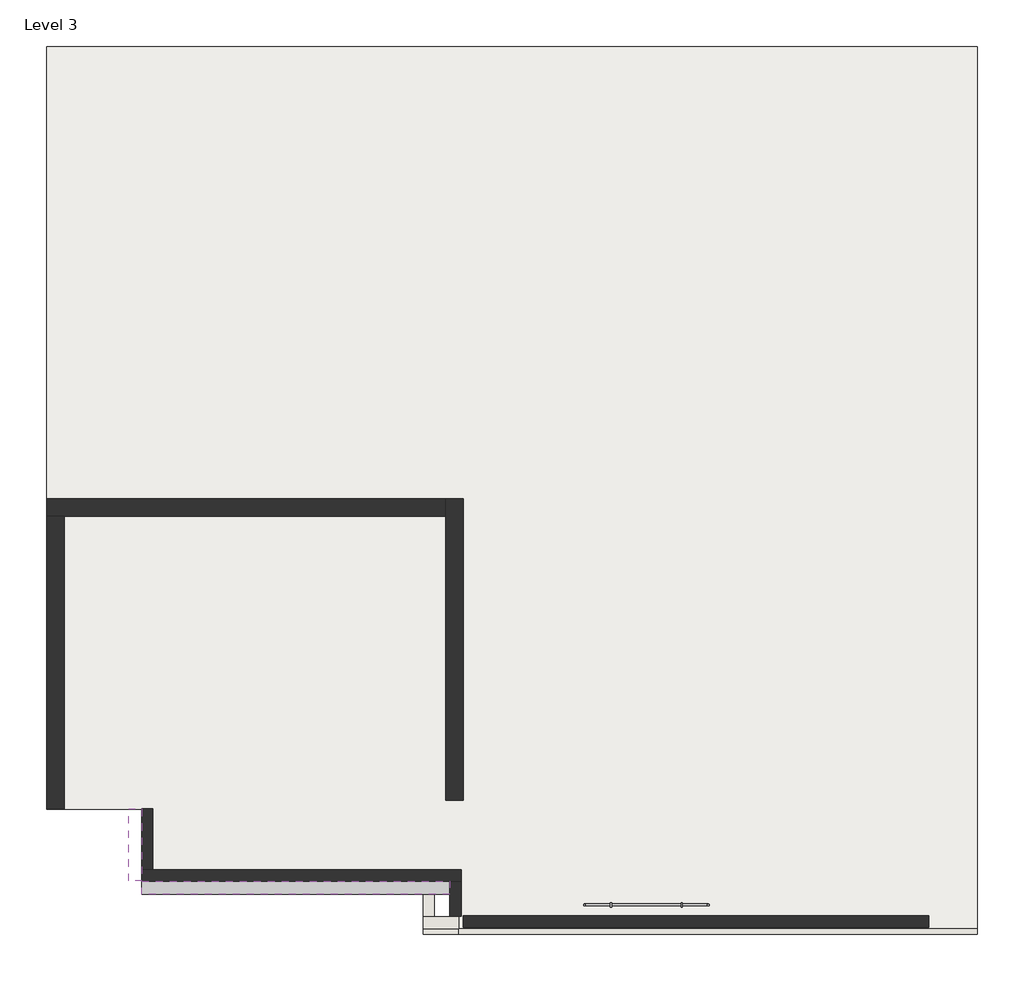
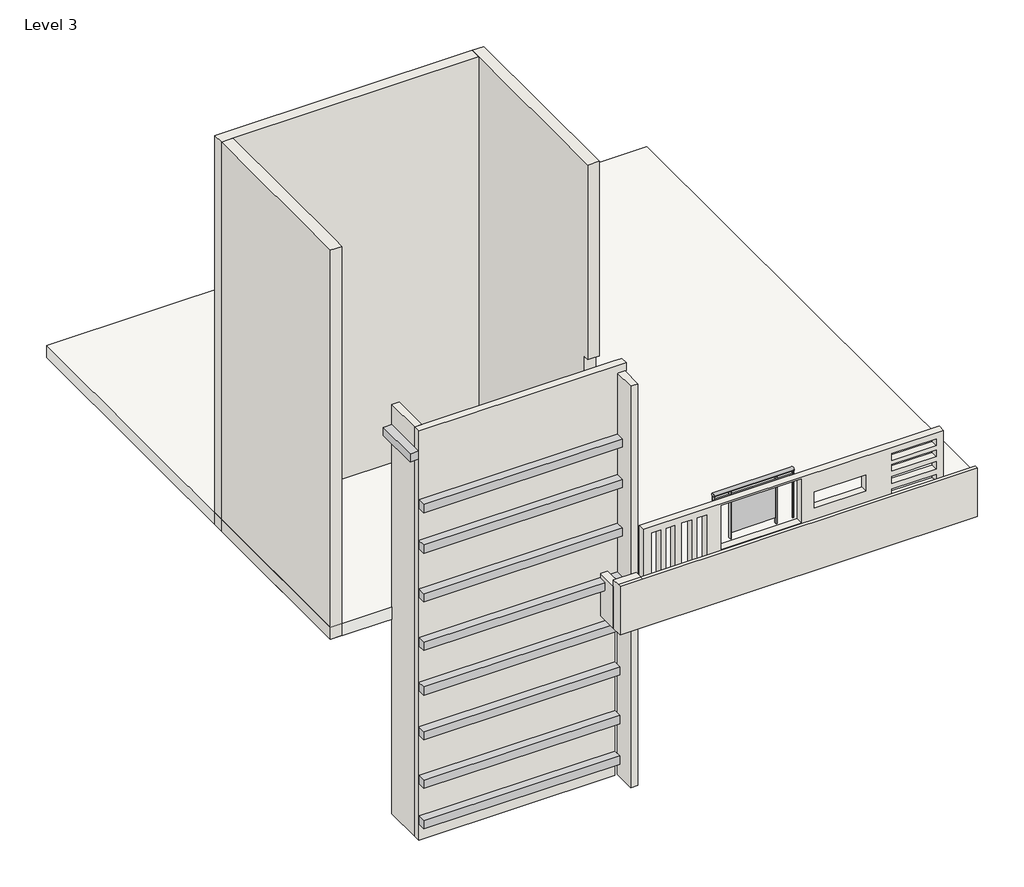
# One storey: 9 proxies, 9 walls, 1 railing, 1 roof.
"""IFC4 building model written with IfcOpenShell, lengths in millimetres."""

from ifc_helpers import new_model, si_unit, point, frame, origin, place, context, project, spatial, polyline, ellipse_curve, trimmed, outline, extrude, faceted_brep, element, save
from ifc_brep_helpers import plane_surface, extruded_surface, advanced_brep

model = new_model("IFC4")

# Units and contexts
model_context = context("Model", 3, world=origin())
ifc_project = project(units=[si_unit("LENGTHUNIT", "METRE", prefix="MILLI")], contexts=[model_context])

# Site, building, storey
site = spatial("IfcSite", under=ifc_project)
building = spatial("IfcBuilding", under=site)
storey = spatial("IfcBuildingStorey", under=building, Name="Level 3", Elevation=7315.2)

# Proxies
placement = place(None, origin())
element("IfcBuildingElementProxy", 1, Name="Cornice", ObjectType="Cornice", at=placement, inside=storey, context=model_context, shape_type="SweptSolid", body=[
    extrude(outline(polyline([(-7613.3936733, 3760.5419215), (-7613.3936733, 3912.9419215), (-4082.7936733, 3912.9419215), (-4082.7936733, 3760.5419215), (-7613.3936733, 3760.5419215)])), frame((0.0, 0.0, 9906.0), z_axis=(0.0, 0.0, 1.0), x_axis=(1.0, 0.0, 0.0)), (0.0, 0.0, 1.0), 152.4),
])
element("IfcBuildingElementProxy", 2, Name="Cornice", ObjectType="Cornice", at=placement, inside=storey, context=model_context, shape_type="SweptSolid", body=[
    extrude(outline(polyline([(-7613.3936733, 3760.5419215), (-7613.3936733, 3912.9419215), (-4082.7936733, 3912.9419215), (-4082.7936733, 3760.5419215), (-7613.3936733, 3760.5419215)])), frame((0.0, 0.0, 9144.0), z_axis=(0.0, 0.0, 1.0), x_axis=(1.0, 0.0, 0.0)), (0.0, 0.0, 1.0), 152.4),
])
element("IfcBuildingElementProxy", 3, Name="Cornice", ObjectType="Cornice", at=placement, inside=storey, context=model_context, shape_type="SweptSolid", body=[
    extrude(outline(polyline([(-7613.3936733, 3760.5419215), (-7613.3936733, 3912.9419215), (-4082.7936733, 3912.9419215), (-4082.7936733, 3760.5419215), (-7613.3936733, 3760.5419215)])), frame((0.0, 0.0, 8229.6), z_axis=(0.0, 0.0, 1.0), x_axis=(1.0, 0.0, 0.0)), (0.0, 0.0, 1.0), 152.4),
])
element("IfcBuildingElementProxy", 4, Name="Cornice", ObjectType="Cornice", at=placement, inside=storey, context=model_context, shape_type="SweptSolid", body=[
    extrude(outline(polyline([(-7613.3936733, 3760.5419215), (-7613.3936733, 3912.9419215), (-4082.7936733, 3912.9419215), (-4082.7936733, 3760.5419215), (-7613.3936733, 3760.5419215)])), frame((0.0, 0.0, 7315.2), z_axis=(0.0, 0.0, 1.0), x_axis=(1.0, 0.0, 0.0)), (0.0, 0.0, 1.0), 152.4),
])
element("IfcBuildingElementProxy", 5, Name="Cornice", ObjectType="Cornice", at=placement, inside=storey, context=model_context, shape_type="SweptSolid", body=[
    extrude(outline(polyline([(-7613.3936733, 3760.5419215), (-7613.3936733, 3912.9419215), (-4133.5936733, 3912.9419215), (-4133.5936733, 3760.5419215), (-7613.3936733, 3760.5419215)])), frame((0.0, 0.0, 6477.1420226), z_axis=(0.0, 0.0, 1.0), x_axis=(1.0, 0.0, 0.0)), (0.0, 0.0, 1.0), 152.4),
])
element("IfcBuildingElementProxy", 6, Name="Cornice", ObjectType="Cornice", at=placement, inside=storey, context=model_context, shape_type="SweptSolid", body=[
    extrude(outline(polyline([(-7613.3936733, 3760.5419215), (-7613.3936733, 3912.9419215), (-4133.5936733, 3912.9419215), (-4133.5936733, 3760.5419215), (-7613.3936733, 3760.5419215)])), frame((0.0, 0.0, 5639.0840451), z_axis=(0.0, 0.0, 1.0), x_axis=(1.0, 0.0, 0.0)), (0.0, 0.0, 1.0), 152.4),
])
element("IfcBuildingElementProxy", 7, Name="Cornice", ObjectType="Cornice", at=placement, inside=storey, context=model_context, shape_type="SweptSolid", body=[
    extrude(outline(polyline([(-7613.3936733, 3760.5419215), (-7613.3936733, 3912.9419215), (-4133.5936733, 3912.9419215), (-4133.5936733, 3760.5419215), (-7613.3936733, 3760.5419215)])), frame((0.0, 0.0, 4724.4), z_axis=(0.0, 0.0, 1.0), x_axis=(1.0, 0.0, 0.0)), (0.0, 0.0, 1.0), 152.4),
])
element("IfcBuildingElementProxy", 8, Name="Cornice", ObjectType="Cornice", at=placement, inside=storey, context=model_context, shape_type="SweptSolid", body=[
    extrude(outline(polyline([(-7613.3936733, 3760.5419215), (-7613.3936733, 3912.9419215), (-4133.5936733, 3912.9419215), (-4133.5936733, 3760.5419215), (-7613.3936733, 3760.5419215)])), frame((0.0, 0.0, 3962.4), z_axis=(0.0, 0.0, 1.0), x_axis=(1.0, 0.0, 0.0)), (0.0, 0.0, 1.0), 152.4),
])
element("IfcBuildingElementProxy", 9, Name="Cornice", ObjectType="Cornice", at=placement, inside=storey, context=model_context, shape_type="SweptSolid", body=[
    extrude(outline(polyline([(-7765.7936733, 4738.4419215), (-7613.3936733, 4738.4419215), (-7613.3936733, 3912.9419215), (-7765.7936733, 3912.9419215), (-7765.7936733, 4738.4419215)])), frame((0.0, 0.0, 10820.4), z_axis=(0.0, 0.0, 1.0), x_axis=(1.0, 0.0, 0.0)), (0.0, 0.0, 1.0), 152.4),
])

# Railing
element("IfcRailing", 10, ObjectType="Glass Panel - Bottom Fill", at=placement, inside=storey, context=model_context, shape_type="SolidModel", body=[
    advanced_brep(
    [(-2542.411491, 3677.9919215, 8534.4), (-2542.411491, 3601.7919215, 8534.4), (-1120.011491, 3677.9919215, 8534.4), (-1120.011491, 3601.7919215, 8534.4)],
    [
        (0, 1, ellipse_curve(frame((-2542.411491, 3639.8919215, 8534.4), z_axis=(-1.0, 0.0, 0.0), x_axis=(0.0, -1.0, 0.0)), 38.1, 28.575)),
        (1, 0, ellipse_curve(frame((-2542.411491, 3639.8919215, 8534.4), z_axis=(-1.0, 0.0, 0.0), x_axis=(0.0, -1.0, 0.0)), 38.1, 28.575)),
        (2, 3, ellipse_curve(frame((-1120.011491, 3639.8919215, 8534.4), z_axis=(1.0, 0.0, 0.0), x_axis=(0.0, -1.0, 0.0)), 38.1, 28.575)),
        (3, 2, ellipse_curve(frame((-1120.011491, 3639.8919215, 8534.4), z_axis=(1.0, 0.0, 0.0), x_axis=(0.0, -1.0, 0.0)), 38.1, 28.575)),
        (0, 2),
        (3, 1),
    ],
    [
        plane_surface(frame((-2542.411491, 3639.8919215, 8534.4), z_axis=(-1.0, 0.0, 0.0), x_axis=(0.0, 1.0, 0.0))),
        plane_surface(frame((-1120.011491, 3639.8919215, 8534.4), z_axis=(1.0, 0.0, 0.0), x_axis=(0.0, 1.0, 0.0))),
        extruded_surface(trimmed(ellipse_curve(frame((-1120.011491, 3639.8919215, 8534.4), z_axis=(-1.0, 0.0, 0.0), x_axis=(0.0, -1.0, 0.0)), 38.1, 28.575), [point((-1120.011491, 3677.9919215, 8534.4))], [point((-1120.011491, 3601.7919215, 8534.4))], True, "CARTESIAN"), (-1422.3999999999999, 0.0, 0.0), 1422.3999999999999),
        extruded_surface(trimmed(ellipse_curve(frame((-1120.011491, 3639.8919215, 8534.4), z_axis=(-1.0, 0.0, 0.0), x_axis=(0.0, -1.0, 0.0)), 38.1, 28.575), [point((-1120.011491, 3601.7919215, 8534.4))], [point((-1120.011491, 3677.9919215, 8534.4))], True, "CARTESIAN"), (-1422.3999999999999, 0.0, 0.0), 1422.3999999999999),
    ],
    [
        (0, [[1, 2]]),
        (1, [[3, 4]]),
        (2, [[-1, 5, -4, 6]]),
        (3, [[-2, -6, -3, -5]]),
    ],
),
    extrude(outline(polyline([(-2542.411491, 3627.1919215), (-2542.411491, 3652.5919215), (-1120.011491, 3652.5919215), (-1120.011491, 3627.1919215), (-2542.411491, 3627.1919215)])), frame((0.0, 0.0, 8420.1), z_axis=(0.0, 0.0, 1.0), x_axis=(1.0, 0.0, 0.0)), (0.0, 0.0, 1.0), 25.4),
    extrude(outline(polyline([(-2542.411491, 3627.1919215), (-2542.411491, 3652.5919215), (-1120.011491, 3652.5919215), (-1120.011491, 3627.1919215), (-2542.411491, 3627.1919215)])), frame((0.0, 0.0, 8318.5), z_axis=(0.0, 0.0, 1.0), x_axis=(1.0, 0.0, 0.0)), (0.0, 0.0, 1.0), 25.4),
    extrude(outline(polyline([(-1431.161491, 3614.4919215), (-1431.161491, 3665.2919215), (-1418.461491, 3665.2919215), (-1418.461491, 3614.4919215), (-1431.161491, 3614.4919215)])), frame((0.0, 0.0, 7620.0), z_axis=(0.0, 0.0, 1.0), x_axis=(1.0, 0.0, 0.0)), (0.0, 0.0, 1.0), 885.6788223),
    extrude(outline(polyline([(-2237.611491, 3646.4270785), (-1424.811491, 3646.4270785), (-1424.811491, 3640.0770785), (-2237.611491, 3640.0770785), (-2237.611491, 3646.4270785)])), frame((0.0, 0.0, 7721.6), z_axis=(0.0, 0.0, 1.0), x_axis=(1.0, 0.0, 0.0)), (0.0, 0.0, 1.0), 596.9),
    extrude(outline(polyline([(-2243.961491, 3614.4919215), (-2243.961491, 3665.2919215), (-2231.261491, 3665.2919215), (-2231.261491, 3614.4919215), (-2243.961491, 3614.4919215)])), frame((0.0, 0.0, 7620.0), z_axis=(0.0, 0.0, 1.0), x_axis=(1.0, 0.0, 0.0)), (0.0, 0.0, 1.0), 885.6788223),
    extrude(outline(polyline([(-1132.711491, 3630.3669215), (-1132.711491, 3649.4169215), (-1113.661491, 3649.4169215), (-1113.661491, 3630.3669215), (-1132.711491, 3630.3669215)])), frame((0.0, 0.0, 7620.0), z_axis=(0.0, 0.0, 1.0), x_axis=(1.0, 0.0, 0.0)), (0.0, 0.0, 1.0), 885.6788223),
    extrude(outline(polyline([(-2548.761491, 3630.3669215), (-2548.761491, 3649.4169215), (-2529.711491, 3649.4169215), (-2529.711491, 3630.3669215), (-2548.761491, 3630.3669215)])), frame((0.0, 0.0, 7620.0), z_axis=(0.0, 0.0, 1.0), x_axis=(1.0, 0.0, 0.0)), (0.0, 0.0, 1.0), 885.6788223),
])

# Roof
element("IfcRoof", 11, ObjectType="Generic - 9\"", at=placement, inside=storey, context=model_context, shape_type="SweptSolid", body=[
    extrude(outline(polyline([(-8705.5936733, 13476.0419215), (1962.4063267, 13476.0419215), (1962.4063267, 3722.4419215), (1962.4063267, 3366.8419215), (-3981.1936733, 3366.8419215), (-3981.1936733, 3976.4419215), (-7486.3936733, 3976.4419215), (-7486.3936733, 4738.4419215), (-8705.5936733, 4738.4419215), (-8705.5936733, 13476.0419215)])), frame((0.0, 0.0, 7315.2), z_axis=(0.0, 0.0, 1.0), x_axis=(1.0, 0.0, 0.0)), (0.0, 0.0, 1.0), 228.6),
])

# Walls
element("IfcWall", 12, ObjectType="Generic - 5\"", at=placement, inside=storey, context=model_context, shape_type="Brep", body=[
    faceted_brep([(-7613.3936733, 3912.9419215, 3657.6), (-4133.5936733, 3912.9419215, 3657.6), (-4133.5936733, 3912.9419215, 7315.2), (-3955.7936733, 3912.9419215, 7315.2), (-3955.7936733, 3912.9419215, 11201.4), (-3930.3936733, 3912.9419215, 11201.4), (-3930.3936733, 3912.9419215, 11349.3315531), (-7613.3936733, 3912.9419215, 11349.3315531), (-7613.3936733, 4039.9419215, 3657.6), (-7613.3936733, 4039.9419215, 11349.3315531), (-7486.3936733, 4039.9419215, 11349.3315531), (-4057.3936733, 4039.9419215, 11349.3315531), (-3930.3936733, 4039.9419215, 11349.3315531), (-3930.3936733, 4039.9419215, 11201.4), (-3955.7936733, 4039.9419215, 11201.4), (-3955.7936733, 4039.9419215, 7315.2), (-4133.5936733, 4039.9419215, 7315.2), (-4133.5936733, 4039.9419215, 3657.6), (-7486.3936733, 4039.9419215, 3657.6)], [[[0, 1, 2, 3, 4, 5, 6, 7]], [[8, 9, 10, 11, 12, 13, 14, 15, 16, 17, 18]], [[1, 0, 8, 18, 17]], [[7, 6, 12, 11, 10, 9]], [[15, 3, 2, 16]], [[1, 17, 16, 2]], [[0, 7, 9, 8]], [[13, 5, 4, 14]], [[4, 3, 15, 14]], [[6, 5, 13, 12]]]),
])
element("IfcWall", 13, ObjectType="Generic - 5\"", at=placement, inside=storey, context=model_context, shape_type="Brep", body=[
    faceted_brep([(-4082.7936733, 3912.9419215, 11201.4), (-4082.7936733, 3912.9419215, 3657.6), (-4082.7936733, 3506.5419215, 3657.6), (-4082.7936733, 3506.5419215, 11201.4), (-3955.7936733, 3912.9419215, 3657.6), (-3955.7936733, 3912.9419215, 7315.2), (-3955.7936733, 3912.9419215, 11201.4), (-3955.7936733, 3506.5419215, 11201.4), (-3955.7936733, 3506.5419215, 3657.6)], [[[0, 1, 2, 3]], [[4, 5, 6, 7, 8]], [[2, 1, 4, 8]], [[0, 3, 7, 6]], [[3, 2, 8, 7]], [[0, 6, 5, 4, 1]]]),
])
element("IfcWall", 14, ObjectType="Generic - 5\"", at=placement, inside=storey, context=model_context, shape_type="Brep", body=[
    faceted_brep([(-7613.3936733, 4738.4419215, 3657.6), (-7613.3936733, 4039.9419215, 3657.6), (-7613.3936733, 4039.9419215, 11349.3315531), (-7613.3936733, 4738.4419215, 11349.3315531), (-7486.3936733, 4738.4419215, 3657.6), (-7486.3936733, 4738.4419215, 10972.8), (-7486.3936733, 4738.4419215, 11349.3315531), (-7486.3936733, 4039.9419215, 11349.3315531), (-7486.3936733, 4039.9419215, 3657.6)], [[[0, 1, 2, 3]], [[4, 5, 6, 7, 8]], [[1, 0, 4, 8]], [[3, 2, 7, 6]], [[2, 1, 8, 7]], [[0, 3, 6, 5, 4]]]),
])
element("IfcWall", 15, ObjectType="Generic - 5\"", at=placement, inside=storey, context=model_context, shape_type="SweptSolid", body=[
    extrude(outline(polyline([(-4261.0195107, 3912.9419215), (-4261.0195107, 3506.5419215), (-4388.0195107, 3506.5419215), (-4388.0195107, 3912.9419215), (-4261.0195107, 3912.9419215)])), frame((0.0, 0.0, 6756.4), z_axis=(0.0, 0.0, 1.0), x_axis=(1.0, 0.0, 0.0)), (0.0, 0.0, 1.0), 787.4),
])
element("IfcWall", 16, ObjectType="Generic - 5\"", at=placement, inside=storey, context=model_context, shape_type="SweptSolid", body=[
    extrude(outline(polyline([(7315.2, -3930.3936733), (7315.2, 1403.6063267), (8525.1410909, 1403.6063267), (8525.1410909, -3930.3936733), (7315.2, -3930.3936733)]), holes=[polyline([(8408.5410475, -3620.6215053), (7417.9410475, -3620.6215053), (7417.9410475, -3773.0215053), (8408.5410475, -3773.0215053), (8408.5410475, -3620.6215053)]), polyline([(8408.5410475, -3364.9892798), (7417.9410475, -3364.9892798), (7417.9410475, -3521.6717373), (8408.5410475, -3521.6717373), (8408.5410475, -3364.9892798)]), polyline([(8408.5410475, -3065.4492875), (7417.9410475, -3065.4492875), (7417.9410475, -3240.5649753), (8408.5410475, -3240.5649753), (8408.5410475, -3065.4492875)]), polyline([(8408.5410475, -2802.7757558), (7417.9410475, -2802.7757558), (7417.9410475, -2968.6748284), (8408.5410475, -2968.6748284), (8408.5410475, -2802.7757558)]), polyline([(8171.6665497, 28.6801951), (7866.8665497, 28.6801951), (7866.8665497, -885.7198049), (8171.6665497, -885.7198049), (8171.6665497, 28.6801951)]), polyline([(8408.5410475, 489.2063267), (8408.5410475, 1276.6063267), (8281.5410475, 1276.6063267), (8281.5410475, 489.2063267), (8408.5410475, 489.2063267)]), polyline([(8202.4002436, 489.2063267), (8202.4002436, 1276.6063267), (8077.9759391, 1276.6063267), (8077.9759391, 489.2063267), (8202.4002436, 489.2063267)]), polyline([(7981.1665497, 489.2063267), (7981.1665497, 1276.6063267), (7843.5690226, 1276.6063267), (7843.5690226, 489.2063267), (7981.1665497, 489.2063267)]), polyline([(7741.123692, 489.2063267), (7741.123692, 1276.6063267), (7610.3830254, 1276.6063267), (7610.3830254, 489.2063267), (7741.123692, 489.2063267)]), polyline([(8497.4410475, -1120.011491), (7671.9410475, -1120.011491), (7671.9410475, -2542.411491), (8497.4410475, -2542.411491), (8497.4410475, -1120.011491)])]), frame((0.0, 3385.8919215, 0.0), z_axis=(0.0, 1.0, 0.0), x_axis=(0.0, 0.0, 1.0)), (0.0, 0.0, 1.0), 127.0),
])
element("IfcWall", 17, ObjectType="Generic - 8\"", at=placement, inside=storey, context=model_context, shape_type="Brep", body=[
    faceted_brep([(-4133.5936733, 8294.4419215, 7315.2), (-4133.5936733, 8091.2419215, 7315.2), (-4133.5936733, 4840.0419215, 7315.2), (-4133.5936733, 4840.0419215, 10972.8), (-4133.5936733, 4738.4419215, 10972.8), (-4133.5936733, 4738.4419215, 14630.4), (-4133.5936733, 4941.6419215, 14630.4), (-4133.5936733, 8091.2419215, 14630.4), (-4133.5936733, 8294.4419215, 14630.4), (-3930.3936733, 8294.4419215, 7315.2), (-3930.3936733, 8294.4419215, 14630.4), (-3930.3936733, 4738.4419215, 14630.4), (-3930.3936733, 4738.4419215, 11349.3315531), (-3930.3936733, 4738.4419215, 10972.8), (-3930.3936733, 4840.0419215, 10972.8), (-3930.3936733, 4840.0419215, 7315.2), (-4057.3936733, 4840.0419215, 10972.8), (-4057.3936733, 4738.4419215, 10972.8)], [[[0, 1, 2, 3, 4, 5, 6, 7, 8]], [[9, 10, 11, 12, 13, 14, 15]], [[2, 1, 0, 9, 15]], [[0, 8, 10, 9]], [[8, 7, 6, 5, 11, 10]], [[3, 2, 15, 14, 16]], [[13, 17, 4, 3, 16, 14]], [[4, 17, 13, 12, 11, 5]]]),
])
element("IfcWall", 18, ObjectType="Generic - 8\"", at=placement, inside=storey, context=model_context, shape_type="Brep", body=[
    faceted_brep([(-4133.5936733, 8294.4419215, 7315.2), (-8705.5936733, 8294.4419215, 7315.2), (-8705.5936733, 8294.4419215, 14630.4), (-4133.5936733, 8294.4419215, 14630.4), (-4133.5936733, 8091.2419215, 7315.2), (-4133.5936733, 8091.2419215, 14630.4), (-8502.3936733, 8091.2419215, 14630.4), (-8705.5936733, 8091.2419215, 14630.4), (-8705.5936733, 8091.2419215, 7315.2), (-8502.3936733, 8091.2419215, 7315.2)], [[[0, 1, 2, 3]], [[4, 5, 6, 7, 8, 9]], [[1, 0, 4, 9, 8]], [[0, 3, 5, 4]], [[2, 1, 8, 7]], [[3, 2, 7, 6, 5]]]),
])
element("IfcWall", 19, ObjectType="Generic - 8\"", at=placement, inside=storey, context=model_context, shape_type="Brep", body=[
    faceted_brep([(-8705.5936733, 8091.2419215, 7315.2), (-8705.5936733, 4738.4419215, 7315.2), (-8705.5936733, 4738.4419215, 14630.4), (-8705.5936733, 8091.2419215, 14630.4), (-8502.3936733, 8091.2419215, 7315.2), (-8502.3936733, 8091.2419215, 14630.4), (-8502.3936733, 4941.6419215, 14630.4), (-8502.3936733, 4738.4419215, 14630.4), (-8502.3936733, 4738.4419215, 10972.8), (-8502.3936733, 4738.4419215, 7315.2)], [[[0, 1, 2, 3]], [[4, 5, 6, 7, 8, 9]], [[1, 0, 4, 9]], [[0, 3, 5, 4]], [[3, 2, 7, 6, 5]], [[1, 9, 8, 7, 2]]]),
])
element("IfcWall", 20, ObjectType="Generic - 8\"", at=placement, inside=storey, context=model_context, shape_type="Brep", body=[
    faceted_brep([(-4388.0195107, 3303.3419215, 6756.4), (1962.4063267, 3303.3419215, 6756.4), (1962.4063267, 3303.3419215, 7670.8), (-3981.1936733, 3303.3419215, 7670.8), (-4388.0195107, 3303.3419215, 7670.8), (-4388.0195107, 3506.5419215, 6756.4), (-4388.0195107, 3506.5419215, 7543.8), (-4388.0195107, 3506.5419215, 7670.8), (-3981.1936733, 3506.5419215, 7670.8), (-3981.1936733, 3506.5419215, 7315.2), (1962.4063267, 3506.5419215, 7315.2), (1962.4063267, 3506.5419215, 6756.4), (-4261.0195107, 3506.5419215, 6756.4), (1962.4063267, 3366.8419215, 7315.2), (1962.4063267, 3366.8419215, 7670.8), (-3981.1936733, 3366.8419215, 7670.8), (-3981.1936733, 3366.8419215, 7315.2), (-4388.0195107, 3366.8419215, 7670.8)], [[[0, 1, 2, 3, 4]], [[5, 6, 7, 8, 9, 10, 11, 12]], [[1, 0, 5, 12, 11]], [[2, 1, 11, 10, 13, 14]], [[15, 14, 13, 16]], [[0, 4, 17, 7, 6, 5]], [[8, 7, 17, 15]], [[8, 15, 16, 9]], [[3, 2, 14, 15]], [[4, 3, 15, 17]], [[13, 10, 9, 16]]]),
])

save(model, "model.ifc")

# Revit data of these elements
# Type "Glass Panel - Bottom Fill"
#   Assembly Code = "C2010400"
#   built-in parameter 1008612 = 0.0416667 (stored number, unit not read)
#   built-in parameter 1008611 = 0.0416667 (stored number, unit not read)
#   built-in parameter 1008609 = 0.333333 (stored number, unit not read)
#   built-in parameter 1008604 = 0.166667 (stored number, unit not read)
#   built-in parameter 1008603 = 0.166667 (stored number, unit not read)
#   Railing Height = 3' - 0"
#   built-in parameter 1008630 = 2
#   built-in parameter 1008610 = 2
#   built-in parameter 1008618 = Baluster - Square : 3/4"
# Type "Generic - 9\""
#   Assembly Code = "B1020"
#   Layers, outside or top first: 0' - 9" no material (function 1)
# Type "Generic - 5\""
#   Assembly Code = "B2010"
#   Layers, outside or top first: 0' - 5" no material (function 1)
# Type "Generic - 8\""
#   Assembly Code = "B2010"
#   Layers, outside or top first: 0' - 8" no material (function 1)
# Elements 1, 2, 3, 4, 5, 6, 7, 8, 9 (IfcBuildingElementProxy, "Cornice")
#   Phase Created = New Construction
#   Materials on its faces: "Default Wall"
# Element 10 (IfcRailing, "Glass Panel - Bottom Fill")
#   built-in parameter 1008621 = 1 (stored number, unit not read)
#   Phase Created = New Construction
#   Materials on its faces: "Glass"
# Element 11 (IfcRoof, "Generic - 9\"")
#   built-in parameter 1001705 = 24.75 (stored number, unit not read)
#   built-in parameter 1001710 = 33615
#   Phase Created = New Construction
#   Materials on its faces: "Default Roof"
# Elements 12, 14 (IfcWall, "Generic - 5\"")
#   built-in parameter 1001111 = -12' - 0"
#   Top Offset = 1' - 2.82408"
#   Base Offset = -12' - 0"
#   wall height = 25' - 2.82408"
#   Phase Created = New Construction
#   Base Constraint = Level 3
#   Top Constraint = Level 4
#   Materials on its faces: "Default Wall"
# Element 13 (IfcWall, "Generic - 5\"")
#   built-in parameter 1001111 = -12' - 0"
#   Top Offset = 0' - 9"
#   Base Offset = -12' - 0"
#   wall height = 24' - 9"
#   Phase Created = New Construction
#   Base Constraint = Level 3
#   Top Constraint = Level 4
#   Materials on its faces: "Default Wall"
# Element 15 (IfcWall, "Generic - 5\"")
#   built-in parameter 1001111 = -1' - 10"
#   Top Offset = -11' - 3"
#   Base Offset = -1' - 10"
#   wall height = 2' - 7"
#   Phase Created = New Construction
#   Base Constraint = Level 3
#   Top Constraint = Level 4
#   Materials on its faces: "Default Wall"
# Element 16 (IfcWall, "Generic - 5\"")
#   Top Offset = -8' - 0.36452"
#   Base Offset = 0' - 0"
#   wall height = 3' - 11.63548"
#   Phase Created = New Construction
#   Base Constraint = Level 3
#   Top Constraint = Level 4
#   Materials on its faces: "Default Wall"
# Elements 17, 18, 19 (IfcWall, "Generic - 8\"")
#   Top Offset = 0' - 0"
#   Base Offset = 0' - 0"
#   Unconnected Height = 24' - 0"
#   wall height = 24' - 0"
#   Phase Created = New Construction
#   Base Constraint = Level 3
#   Materials on its faces: "Default Wall"
# Element 20 (IfcWall, "Generic - 8\"")
#   built-in parameter 1001111 = -1' - 10"
#   Top Offset = 0' - 0"
#   Base Offset = -1' - 10"
#   Unconnected Height = 3' - 0"
#   wall height = 3' - 0"
#   Phase Created = New Construction
#   Base Constraint = Level 3
#   Materials on its faces: "Default Wall"
# Materials
#   "Default Wall": colour RGB 128 128 128, transparency 0
#   "Glass": class "Glass", colour RGB 0 128 192, transparency 0.75, Description = "Soda Lime Glass", Cost = 0
#   "Default Roof": colour RGB 88 101 114, transparency 0
